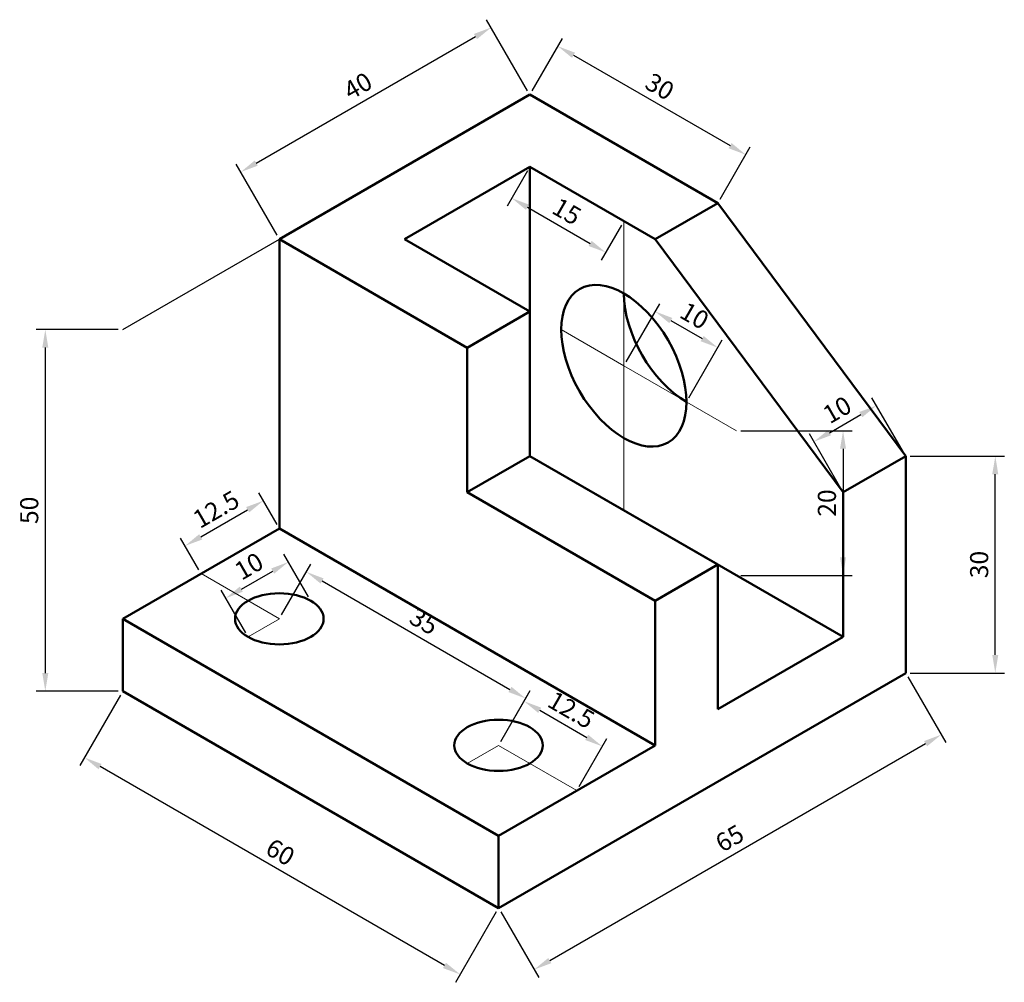
# Model space of a CAD drawing. Units: millimetres. Extents: x 340 to 477, y 198 to 331.
import ezdxf

# ---------------------------------------------------------------- set-up
doc = ezdxf.new("R2010")
doc.units = ezdxf.units.MM
doc.linetypes.add('CENTER', pattern=[50.8, 31.75, -6.35, 6.35, -6.35])
for name, color, linetype, lineweight in [('M-CNTR', 4, 'CENTER', 18), ('M-DIMS', 2, 'Continuous', 25), ('M-OUTL', 7, 'Continuous', 50)]:
    doc.layers.add(name, color=color, linetype=linetype, lineweight=lineweight)
doc.styles.get("Standard").update_dxf_attribs({"font": 'arial.ttf'})
doc.dimstyles.new('ISO-25', dxfattribs={"dimtxt": 2.5, "dimasz": 2.5, "dimexe": 1.25, "dimexo": 0.625, "dimtad": 1, "dimdsep": 46, "dimtxsty": 'Standard', "dimcen": 2.5, "dimadec": 0, "dimazin": 0, "dimtfac": 1, "dimtmove": 0, "dimatfit": 3, "dimfxl": 1, "dimarcsym": 0})

# ---------------------------------------------------------------- blocks, each defined once
blk = doc.blocks.new('*D1')
at = {"layer": 'Defpoints', "color": 0, "transparency": 16777216}
for p in [(354.66, 238.02), (349.36, 228.83), (406.62, 208.02)]:
    blk.add_point(p, dxfattribs=at)
at = {"layer": 'M-DIMS', "color": 0, "lineweight": -2, "transparency": 16777216}
for p, q in [((354.35, 237.48), (348.73, 227.74)), ((399.15, 200.08), (351.52, 227.58)), ((406.31, 207.48), (400.69, 197.74))]:
    blk.add_line(p, q, dxfattribs=at)
at = {"layer": 'M-DIMS', "color": 0, "transparency": 16777216}
for points in [[(351.73, 227.94), (351.31, 227.21), (349.36, 228.83)], [(399.36, 200.44), (398.94, 199.71), (401.32, 198.83)]]:
    blk.add_solid(points, dxfattribs=at)
at = {"layer": 'M-DIMS', "color": 0, "transparency": 16777216, "insert": (376.29, 215.47), "char_height": 2.5, "attachment_point": 5, "rotation": 330}
blk.add_mtext('60', dxfattribs=at)
blk = doc.blocks.new('*D2')
at = {"layer": 'Defpoints', "color": 0, "transparency": 16777216}
for p in [(462.92, 240.52), (467.84, 232), (406.62, 208.02)]:
    blk.add_point(p, dxfattribs=at)
at = {"layer": 'M-DIMS', "color": 0, "lineweight": -2, "transparency": 16777216}
for p, q in [((463.23, 239.98), (468.46, 230.91)), ((413.71, 200.75), (465.67, 230.75)), ((406.94, 207.48), (412.17, 198.41))]:
    blk.add_line(p, q, dxfattribs=at)
at = {"layer": 'M-DIMS', "color": 0, "transparency": 16777216}
for points in [[(465.46, 231.11), (465.88, 230.39), (467.84, 232)], [(413.5, 201.11), (413.92, 200.39), (411.54, 199.5)]]:
    blk.add_solid(points, dxfattribs=at)
at = {"layer": 'M-DIMS', "color": 0, "transparency": 16777216, "insert": (438.74, 217.39), "char_height": 2.5, "attachment_point": 5, "rotation": 30}
blk.add_mtext('65', dxfattribs=at)
blk = doc.blocks.new('*D3')
at = {"layer": 'Defpoints', "color": 0, "transparency": 16777216}
for p in [(458.88, 277.51), (462.92, 270.52), (454.26, 265.52)]:
    blk.add_point(p, dxfattribs=at)
at = {"layer": 'M-DIMS', "color": 0, "lineweight": -2, "transparency": 16777216}
for p, q in [((462.6, 271.06), (458.26, 278.59)), ((452.39, 273.76), (456.72, 276.26)), ((453.94, 266.06), (449.6, 273.59))]:
    blk.add_line(p, q, dxfattribs=at)
at = {"layer": 'M-DIMS', "color": 0, "transparency": 16777216}
for points in [[(456.51, 276.62), (456.92, 275.9), (458.88, 277.51)], [(452.18, 274.12), (452.59, 273.4), (450.22, 272.51)]]:
    blk.add_solid(points, dxfattribs=at)
at = {"layer": 'M-DIMS', "color": 0, "transparency": 16777216, "insert": (453.6, 276.65), "char_height": 2.5, "attachment_point": 5, "rotation": 30}
blk.add_mtext('10', dxfattribs=at)
blk = doc.blocks.new('*D4')
at = {"layer": 'Defpoints', "color": 0, "transparency": 16777216}
for p in [(462.92, 270.52), (475.31, 270.52), (462.92, 240.52)]:
    blk.add_point(p, dxfattribs=at)
at = {"layer": 'M-DIMS', "color": 0, "lineweight": -2, "transparency": 16777216}
for p, q in [((463.54, 270.52), (476.56, 270.52)), ((475.31, 243.02), (475.31, 268.02)), ((463.54, 240.52), (476.56, 240.52))]:
    blk.add_line(p, q, dxfattribs=at)
at = {"layer": 'M-DIMS', "color": 0, "transparency": 16777216}
for points in [[(474.89, 268.02), (475.72, 268.02), (475.31, 270.52)], [(474.89, 243.02), (475.72, 243.02), (475.31, 240.52)]]:
    blk.add_solid(points, dxfattribs=at)
at = {"layer": 'M-DIMS', "color": 0, "transparency": 16777216, "insert": (473.4, 255.52), "char_height": 2.5, "attachment_point": 5, "rotation": 90}
blk.add_mtext('30', dxfattribs=at)
blk = doc.blocks.new('*D5')
at = {"layer": 'Defpoints', "color": 0, "transparency": 16777216}
for p in [(405.6, 329.8), (410.95, 320.52), (376.31, 300.52)]:
    blk.add_point(p, dxfattribs=at)
at = {"layer": 'M-DIMS', "color": 0, "lineweight": -2, "transparency": 16777216}
for p, q in [((410.64, 321.06), (404.97, 330.88)), ((373.12, 311.05), (403.43, 328.55)), ((376, 301.06), (370.33, 310.88))]:
    blk.add_line(p, q, dxfattribs=at)
at = {"layer": 'M-DIMS', "color": 0, "transparency": 16777216}
for points in [[(403.22, 328.91), (403.64, 328.19), (405.6, 329.8)], [(372.91, 311.41), (373.33, 310.69), (370.96, 309.8)]]:
    blk.add_solid(points, dxfattribs=at)
at = {"layer": 'M-DIMS', "color": 0, "transparency": 16777216, "insert": (387.33, 321.44), "char_height": 2.5, "attachment_point": 5, "rotation": 30}
blk.add_mtext('40', dxfattribs=at)
blk = doc.blocks.new('*D6')
at = {"layer": 'Defpoints', "color": 0, "transparency": 16777216}
for p in [(410.95, 320.52), (440.8, 312.21), (436.94, 305.52)]:
    blk.add_point(p, dxfattribs=at)
at = {"layer": 'M-DIMS', "color": 0, "lineweight": -2, "transparency": 16777216}
for p, q in [((411.27, 321.06), (415.45, 328.3)), ((416.99, 325.96), (438.64, 313.46)), ((437.25, 306.06), (441.43, 313.3))]:
    blk.add_line(p, q, dxfattribs=at)
at = {"layer": 'M-DIMS', "color": 0, "transparency": 16777216}
for points in [[(417.19, 326.32), (416.78, 325.6), (414.82, 327.21)], [(438.84, 313.82), (438.43, 313.1), (440.8, 312.21)]]:
    blk.add_solid(points, dxfattribs=at)
at = {"layer": 'M-DIMS', "color": 0, "transparency": 16777216, "insert": (428.76, 321.36), "char_height": 2.5, "attachment_point": 5, "rotation": 330}
blk.add_mtext('30', dxfattribs=at)
blk = doc.blocks.new('*D7')
at = {"layer": 'Defpoints', "color": 0, "transparency": 16777216}
for p in [(376.31, 248.02), (410.37, 237), (406.62, 230.52)]:
    blk.add_point(p, dxfattribs=at)
at = {"layer": 'M-DIMS', "color": 0, "lineweight": -2, "transparency": 16777216}
for p, q in [((376.63, 248.56), (380.68, 255.58)), ((382.22, 253.25), (408.2, 238.25)), ((406.94, 231.06), (410.99, 238.08))]:
    blk.add_line(p, q, dxfattribs=at)
at = {"layer": 'M-DIMS', "color": 0, "transparency": 16777216}
for points in [[(382.43, 253.61), (382.01, 252.89), (380.06, 254.5)], [(408.41, 238.61), (407.99, 237.89), (410.37, 237)]]:
    blk.add_solid(points, dxfattribs=at)
at = {"layer": 'M-DIMS', "color": 0, "transparency": 16777216, "insert": (396.16, 247.4), "char_height": 2.5, "attachment_point": 5, "rotation": 330}
blk.add_mtext('35', dxfattribs=at)
blk = doc.blocks.new('*D8')
at = {"layer": 'Defpoints', "color": 0, "transparency": 16777216}
for p in [(354.66, 288.02), (343.95, 238.02), (354.66, 238.02)]:
    blk.add_point(p, dxfattribs=at)
at = {"layer": 'M-DIMS', "color": 0, "lineweight": -2, "transparency": 16777216}
for p, q in [((354.04, 288.02), (342.7, 288.02)), ((343.95, 285.52), (343.95, 240.52)), ((354.04, 238.02), (342.7, 238.02))]:
    blk.add_line(p, q, dxfattribs=at)
at = {"layer": 'M-DIMS', "color": 0, "transparency": 16777216}
for points in [[(343.53, 285.52), (344.37, 285.52), (343.95, 288.02)], [(343.53, 240.52), (344.37, 240.52), (343.95, 238.02)]]:
    blk.add_solid(points, dxfattribs=at)
at = {"layer": 'M-DIMS', "color": 0, "transparency": 16777216, "insert": (342.05, 263.02), "char_height": 2.5, "attachment_point": 5, "rotation": 90}
blk.add_mtext('50', dxfattribs=at)
blk = doc.blocks.new('*D9')
at = {"layer": 'Defpoints', "color": 0, "transparency": 16777216}
for p in [(410.95, 310.52), (423.94, 303.02), (421.45, 298.69)]:
    blk.add_point(p, dxfattribs=at)
at = {"layer": 'M-DIMS', "color": 0, "lineweight": -2, "transparency": 16777216}
for p, q in [((410.64, 309.98), (407.83, 305.11)), ((410.62, 304.94), (419.28, 299.94)), ((423.63, 302.48), (420.82, 297.61))]:
    blk.add_line(p, q, dxfattribs=at)
at = {"layer": 'M-DIMS', "color": 0, "transparency": 16777216}
for points in [[(410.83, 305.3), (410.41, 304.58), (408.46, 306.19)], [(419.49, 300.3), (419.07, 299.58), (421.45, 298.69)]]:
    blk.add_solid(points, dxfattribs=at)
at = {"layer": 'M-DIMS', "color": 0, "transparency": 16777216, "insert": (415.9, 304.08), "char_height": 2.5, "attachment_point": 5, "rotation": 330}
blk.add_mtext('15', dxfattribs=at)
blk = doc.blocks.new('*D10')
at = {"layer": 'Defpoints', "color": 0, "transparency": 16777216}
for p in [(439.51, 274.03), (439.51, 254.03), (454.26, 254.03)]:
    blk.add_point(p, dxfattribs=at)
at = {"layer": 'M-DIMS', "color": 0, "lineweight": -2, "transparency": 16777216}
for p, q in [((440.14, 274.03), (455.51, 274.03)), ((454.26, 271.53), (454.26, 256.53)), ((440.14, 254.03), (455.51, 254.03))]:
    blk.add_line(p, q, dxfattribs=at)
at = {"layer": 'M-DIMS', "color": 0, "transparency": 16777216}
for points in [[(453.84, 271.53), (454.67, 271.53), (454.26, 274.03)], [(453.84, 256.53), (454.67, 256.53), (454.26, 254.03)]]:
    blk.add_solid(points, dxfattribs=at)
at = {"layer": 'M-DIMS', "color": 0, "transparency": 16777216, "insert": (452.35, 264.03), "char_height": 2.5, "attachment_point": 5, "rotation": 90}
blk.add_mtext('20', dxfattribs=at)
blk = doc.blocks.new('*D11')
at = {"layer": 'Defpoints', "color": 0, "transparency": 16777216}
for p in [(377.55, 255.87), (380.64, 250.52), (371.98, 245.52)]:
    blk.add_point(p, dxfattribs=at)
at = {"layer": 'M-DIMS', "color": 0, "lineweight": -2, "transparency": 16777216}
for p, q in [((380.33, 251.06), (376.93, 256.96)), ((371.06, 252.12), (375.39, 254.62)), ((371.67, 246.06), (368.27, 251.96))]:
    blk.add_line(p, q, dxfattribs=at)
at = {"layer": 'M-DIMS', "color": 0, "transparency": 16777216}
for points in [[(375.18, 254.98), (375.59, 254.26), (377.55, 255.87)], [(370.85, 252.48), (371.26, 251.76), (368.89, 250.87)]]:
    blk.add_solid(points, dxfattribs=at)
at = {"layer": 'M-DIMS', "color": 0, "transparency": 16777216, "insert": (372.27, 255.02), "char_height": 2.5, "attachment_point": 5, "rotation": 30}
blk.add_mtext('10', dxfattribs=at)
blk = doc.blocks.new('*D12')
at = {"layer": 'Defpoints', "color": 0, "transparency": 16777216}
for p in [(374.1, 264.35), (376.31, 260.52), (365.49, 254.27)]:
    blk.add_point(p, dxfattribs=at)
at = {"layer": 'M-DIMS', "color": 0, "lineweight": -2, "transparency": 16777216}
for p, q in [((376, 261.06), (373.47, 265.44)), ((365.44, 259.35), (371.93, 263.1)), ((365.18, 254.81), (362.65, 259.19))]:
    blk.add_line(p, q, dxfattribs=at)
at = {"layer": 'M-DIMS', "color": 0, "transparency": 16777216}
for points in [[(371.72, 263.47), (372.14, 262.74), (374.1, 264.35)], [(365.23, 259.72), (365.65, 258.99), (363.27, 258.1)]]:
    blk.add_solid(points, dxfattribs=at)
at = {"layer": 'M-DIMS', "color": 0, "transparency": 16777216, "insert": (367.73, 262.88), "char_height": 2.5, "attachment_point": 5, "rotation": 30}
blk.add_mtext('12.5', dxfattribs=at)
blk = doc.blocks.new('*D13')
at = {"layer": 'Defpoints', "color": 0, "transparency": 16777216}
for p in [(406.62, 230.52), (420.97, 230.37), (417.45, 224.27)]:
    blk.add_point(p, dxfattribs=at)
at = {"layer": 'M-DIMS', "color": 0, "lineweight": -2, "transparency": 16777216}
for p, q in [((406.94, 231.06), (410.77, 237.7)), ((412.31, 235.37), (418.81, 231.62)), ((417.76, 224.81), (421.6, 231.45))]:
    blk.add_line(p, q, dxfattribs=at)
at = {"layer": 'M-DIMS', "color": 0, "transparency": 16777216}
for points in [[(412.52, 235.73), (412.1, 235.01), (410.15, 236.62)], [(419.02, 231.98), (418.6, 231.26), (420.97, 230.37)]]:
    blk.add_solid(points, dxfattribs=at)
at = {"layer": 'M-DIMS', "color": 0, "transparency": 16777216, "insert": (416.51, 235.14), "char_height": 2.5, "attachment_point": 5, "rotation": 330}
blk.add_mtext('12.5', dxfattribs=at)
blk = doc.blocks.new('*D14')
at = {"layer": 'Defpoints', "color": 0, "transparency": 16777216}
for p in [(436.94, 285.52), (423.94, 283.02), (432.61, 278.02)]:
    blk.add_point(p, dxfattribs=at)
at = {"layer": 'M-DIMS', "color": 0, "lineweight": -2, "transparency": 16777216}
for p, q in [((424.26, 283.56), (428.9, 291.6)), ((430.44, 289.27), (434.77, 286.77)), ((432.92, 278.56), (437.56, 286.6))]:
    blk.add_line(p, q, dxfattribs=at)
at = {"layer": 'M-DIMS', "color": 0, "transparency": 16777216}
for points in [[(430.65, 289.63), (430.23, 288.91), (428.28, 290.52)], [(434.98, 287.13), (434.56, 286.41), (436.94, 285.52)]]:
    blk.add_solid(points, dxfattribs=at)
at = {"layer": 'M-DIMS', "color": 0, "transparency": 16777216, "insert": (433.56, 289.66), "char_height": 2.5, "attachment_point": 5, "rotation": 330}
blk.add_mtext('10', dxfattribs=at)

msp = doc.modelspace()

# ---------------------------------------------------------------- linework, layer by layer
at = {"layer": 'M-CNTR'}
for p, q in [((423.945, 283.017), (423.945, 303.017)), ((423.945, 293.017), (423.945, 283.017)), ((423.945, 283.017), (415.285, 288.017)), ((423.945, 283.017), (423.945, 263.017)), ((423.945, 283.017), (439.512, 274.029)), ((376.314, 248.017), (365.488, 254.267)), ((376.314, 248.017), (371.983, 245.517)), ((406.624, 230.517), (402.294, 228.017)), ((406.624, 230.517), (417.45, 224.267))]:
    msp.add_line(p, q, dxfattribs=at)
at = {"layer": 'M-DIMS'}
msp.add_line((354.663, 288.017), (376.314, 300.517), dxfattribs=at)
at = {"layer": 'M-OUTL'}
for p, q in [((376.314, 300.517), (410.955, 320.517)), ((410.955, 320.517), (436.935, 305.517)), ((393.634, 300.517), (410.955, 310.517)), ((410.955, 310.517), (428.275, 300.517)), ((410.955, 310.517), (410.955, 270.517)), ((428.275, 300.517), (436.935, 305.517)), ((436.935, 305.517), (462.916, 270.517)), ((376.314, 260.517), (376.314, 300.517)), ((376.314, 300.517), (402.294, 285.517)), ((410.955, 290.517), (393.634, 300.517)), ((428.275, 300.517), (454.256, 265.517)), ((402.294, 285.517), (410.955, 290.517)), ((410.955, 290.517), (410.955, 270.517)), ((402.294, 285.517), (402.294, 265.517)), ((402.294, 265.517), (410.955, 270.517)), ((410.955, 270.517), (436.935, 255.517)), ((454.256, 245.517), (410.955, 270.517)), ((462.916, 270.517), (454.256, 265.517)), ((462.916, 240.517), (462.916, 270.517)), ((402.294, 265.517), (428.275, 250.517)), ((454.256, 265.517), (454.256, 245.517)), ((354.663, 248.017), (376.314, 260.517)), ((376.314, 260.517), (428.275, 230.517)), ((436.935, 255.517), (428.275, 250.517)), ((436.935, 235.517), (436.935, 255.517)), ((428.275, 250.517), (428.275, 230.517)), ((406.624, 218.017), (354.663, 248.017)), ((354.663, 248.017), (354.663, 238.017)), ((454.256, 245.517), (436.935, 235.517)), ((406.624, 208.017), (462.916, 240.517)), ((406.624, 208.017), (354.663, 238.017)), ((428.275, 230.517), (406.624, 218.017)), ((406.624, 218.017), (406.624, 208.017))]:
    msp.add_line(p, q, dxfattribs=at)
for centre, major_axis in [((423.945, 283.017), (6.124, -10.607)), ((376.314, 248.017), (-6.124, 0)), ((406.624, 230.517), (-6.124, 0))]:
    msp.add_ellipse(centre, major_axis=major_axis, ratio=0.5773503, dxfattribs=at)
msp.add_ellipse((432.605, 288.017), major_axis=(6.124, -10.607), ratio=0.5773503, start_param=3.9269908, end_param=5.4977871, dxfattribs=at)

# ---------------------------------------------------------------- dimensions: what is measured, and where the dimension line sits
at = {"layer": 'M-DIMS'}
for p1, p2, distance, picture, middle in [((376.314, 300.517), (410.955, 320.517), 10.716, '*D5', (387.325, 321.444)), ((410.955, 320.517), (436.935, 305.517), 7.732, '*D6', (428.762, 321.36)), ((410.955, 310.517), (423.945, 303.017), -4.998, '*D9', (415.901, 304.085)), ((423.945, 283.017), (432.605, 278.017), 8.66, '*D14', (433.556, 289.663)), ((454.256, 265.517), (462.916, 270.517), 8.071, '*D3', (453.6, 276.653)), ((365.488, 254.267), (376.314, 260.517), 4.432, '*D12', (367.734, 262.876)), ((371.983, 245.517), (380.644, 250.517), 6.186, '*D11', (372.27, 255.02)), ((376.314, 248.017), (406.624, 230.517), 7.487, '*D7', (396.164, 247.398)), ((406.624, 208.017), (462.916, 240.517), -9.838, '*D2', (438.739, 217.393)), ((406.624, 208.017), (354.663, 238.017), 10.613, '*D1', (376.288, 215.472)), ((406.624, 230.517), (417.45, 224.267), 7.047, '*D13', (416.511, 235.141))]:
    dim = msp.add_aligned_dim(p1=p1, p2=p2, distance=distance, dimstyle='ISO-25', override={"dimclrd": 0, "dimclre": 0, "dimclrt": 0}, dxfattribs=at)
    dim.commit()
    dim.dimension.update_dxf_attribs({"geometry": picture, "text_midpoint": middle})
for base, p1, p2, picture, middle in [((343.949, 238.017), (354.663, 288.017), (354.663, 238.017), '*D8', (342.048, 263.017)), ((454.256, 254.029), (439.512, 274.029), (439.512, 254.029), '*D10', (452.354, 264.029)), ((475.305, 270.517), (462.916, 240.517), (462.916, 270.517), '*D4', (473.403, 255.517))]:
    dim = msp.add_linear_dim(base=base, p1=p1, p2=p2, angle=90, dimstyle='ISO-25', override={"dimclrd": 0, "dimclre": 0, "dimclrt": 0}, dxfattribs=at)
    dim.commit()
    dim.dimension.update_dxf_attribs({"geometry": picture, "text_midpoint": middle})

doc.saveas('drawing.dxf')
